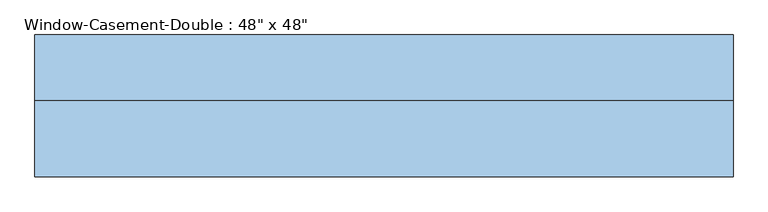
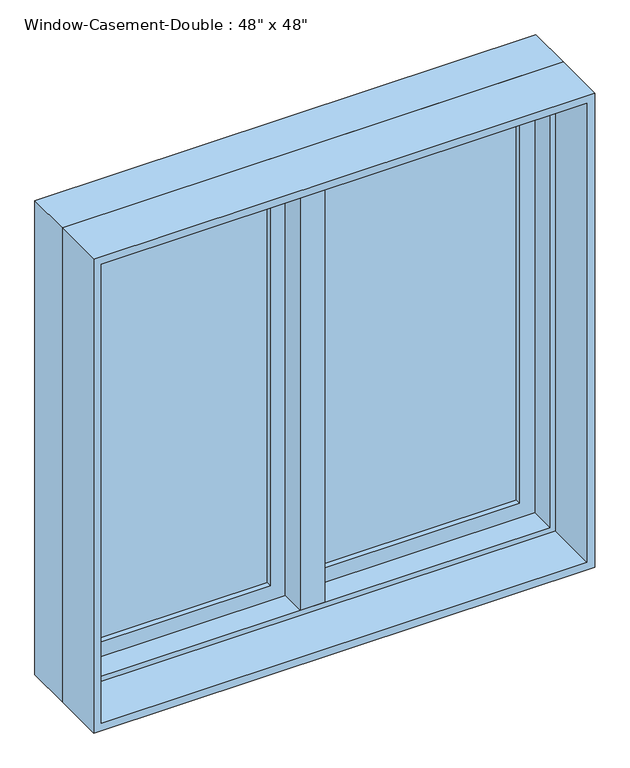
"""IFC4 building model written with IfcOpenShell, lengths in millimetres: window geometry."""

from ifc_helpers import new_model, si_unit, frame, origin, place, context, project, spatial, polyline, outline, extrude, faceted_brep, source, transform, mapped, element, save


def window_9200f5ac(model_context):
    return source(origin(), model_context, "Body", "SolidModel", [
        faceted_brep([(577.85, 82.55, 2101.85), (577.85, 19.05, 2101.85), (-577.85, 19.05, 2101.85), (-577.85, 82.55, 2101.85), (596.9, 133.35, 2120.9), (596.9, 82.55, 2120.9), (-596.9, 82.55, 2120.9), (-596.9, 133.35, 2120.9), (609.6, 19.05, 2133.6), (609.6, 133.35, 2133.6), (-609.6, 133.35, 2133.6), (-609.6, 19.05, 2133.6), (-577.85, 19.05, 946.15), (-577.85, 82.55, 946.15), (-596.9, 82.55, 927.1), (-596.9, 133.35, 927.1), (-609.6, 133.35, 914.4), (-609.6, 19.05, 914.4), (577.85, 19.05, 946.15), (577.85, 82.55, 946.15), (596.9, 82.55, 927.1), (596.9, 133.35, 927.1), (609.6, 133.35, 914.4), (609.6, 19.05, 914.4)], [[[0, 1, 2, 3]], [[4, 5, 6, 7]], [[8, 9, 10, 11]], [[3, 2, 12, 13]], [[7, 6, 14, 15]], [[11, 10, 16, 17]], [[13, 12, 18, 19]], [[15, 14, 20, 21]], [[17, 16, 22, 23]], [[11, 17, 23, 8], [1, 18, 12, 2]], [[19, 18, 1, 0]], [[5, 20, 14, 6], [3, 13, 19, 0]], [[21, 20, 5, 4]], [[23, 22, 9, 8]], [[9, 22, 16, 10], [7, 15, 21, 4]]]),
        extrude(outline(polyline([(2133.6, -609.6), (914.4, -609.6), (914.4, 609.6), (2133.6, 609.6), (2133.6, -609.6)]), holes=[polyline([(2114.55, 590.55), (933.45, 590.55), (933.45, -590.55), (2114.55, -590.55), (2114.55, 590.55)])]), frame((0.0, -114.3, 0.0), z_axis=(0.0, 1.0, 0.0), x_axis=(0.0, 0.0, 1.0)), (0.0, 0.0, 1.0), 133.35),
        extrude(outline(polyline([(927.1, 596.9), (2120.9, 596.9), (2120.9, 9.525), (927.1, 9.525), (927.1, 596.9)]), holes=[polyline([(984.25, 66.675), (2063.75, 66.675), (2063.75, 539.75), (984.25, 539.75), (984.25, 66.675)])]), frame((0.0, 82.55, 0.0), z_axis=(0.0, 1.0, 0.0), x_axis=(0.0, 0.0, 1.0)), (0.0, 0.0, 1.0), 44.45),
        extrude(outline(polyline([(2120.9, -596.9), (927.1, -596.9), (927.1, -9.525), (2120.9, -9.525), (2120.9, -596.9)]), holes=[polyline([(2063.75, -66.675), (984.25, -66.675), (984.25, -539.75), (2063.75, -539.75), (2063.75, -66.675)])]), frame((0.0, 82.55, 0.0), z_axis=(0.0, 1.0, 0.0), x_axis=(0.0, 0.0, 1.0)), (0.0, 0.0, 1.0), 44.45),
        extrude(outline(polyline([(539.75, 114.3), (539.75, 107.95), (66.675, 107.95), (66.675, 114.3), (539.75, 114.3)])), frame((0.0, 0.0, 984.25), z_axis=(0.0, 0.0, 1.0), x_axis=(1.0, 0.0, 0.0)), (0.0, 0.0, 1.0), 1079.5),
        extrude(outline(polyline([(66.675, 95.25), (66.675, 101.6), (539.75, 101.6), (539.75, 95.25), (66.675, 95.25)])), frame((0.0, 0.0, 984.25), z_axis=(0.0, 0.0, 1.0), x_axis=(1.0, 0.0, 0.0)), (0.0, 0.0, 1.0), 1079.5),
        extrude(outline(polyline([(-66.675, 114.3), (-66.675, 107.95), (-539.75, 107.95), (-539.75, 114.3), (-66.675, 114.3)])), frame((0.0, 0.0, 984.25), z_axis=(0.0, 0.0, 1.0), x_axis=(1.0, 0.0, 0.0)), (0.0, 0.0, 1.0), 1079.5),
        extrude(outline(polyline([(-539.75, 95.25), (-539.75, 101.6), (-66.675, 101.6), (-66.675, 95.25), (-539.75, 95.25)])), frame((0.0, 0.0, 984.25), z_axis=(0.0, 0.0, 1.0), x_axis=(1.0, 0.0, 0.0)), (0.0, 0.0, 1.0), 1079.5),
        faceted_brep([(9.525, 133.35, 2120.9), (-9.525, 133.35, 2120.9), (-9.525, 82.55, 2120.9), (9.525, 82.55, 2120.9), (9.525, 133.35, 927.1), (9.525, 82.55, 927.1), (-9.525, 82.55, 927.1), (-9.525, 133.35, 927.1), (-9.525, 82.55, 946.15), (-9.525, 82.55, 2101.85), (-30.1625, 82.55, 946.15), (-30.1625, 82.55, 2101.85), (-30.1625, 19.05, 946.15), (-30.1625, 19.05, 2101.85), (30.1625, 19.05, 946.15), (30.1625, 19.05, 2101.85), (30.1625, 82.55, 946.15), (30.1625, 82.55, 2101.85), (9.525, 82.55, 946.15), (9.525, 82.55, 2101.85)], [[[0, 1, 2, 3]], [[4, 5, 6, 7]], [[1, 0, 4, 7]], [[2, 1, 7, 6, 8, 9]], [[9, 8, 10, 11]], [[11, 10, 12, 13]], [[13, 12, 14, 15]], [[15, 14, 16, 17]], [[17, 16, 18, 19]], [[0, 3, 19, 18, 5, 4]], [[18, 8, 6, 5]], [[9, 19, 3, 2]], [[8, 18, 16, 14, 12, 10]], [[19, 9, 11, 13, 15, 17]]]),
    ])


if __name__ == "__main__":
    model = new_model("IFC4")
    model_context = context("Model", 3, world=origin())
    ifc_project = project(units=[si_unit("LENGTHUNIT", "METRE", prefix="MILLI")], contexts=[model_context])
    site = spatial("IfcSite", under=ifc_project)
    building = spatial("IfcBuilding", under=site)
    placement = place(None, origin())
    window_shape = window_9200f5ac(model_context)
    element("IfcWindow", 1, ObjectType="Window-Casement-Double : 48\" x 48\"", at=placement, inside=building, context=model_context, shape_type="MappedRepresentation", body=[
        mapped(window_shape, transform((0.0, 0.0, 0.0), x_axis=(1.0, 0.0, 0.0), y_axis=(0.0, 1.0, 0.0), z_axis=(0.0, 0.0, 1.0))),
    ])
    save(model, "model.ifc")

# Revit data of these elements
# Type "Window-Casement-Double : 48\" x 48\""
#   Type Mark = "18"
#   Fire Rating = "0.5h"
#   Assembly Code = "B2020100"
#   Analytic Construction = "Double glazing - domestic"
#   Frame Extension [instance default] = 0' - 0 1/4"
#   Window Inset [instance default] = 0' - 0"
#   Wall Thickness [instance default] = 0' - 6"
#   Interior Wall Closure [instance default] = 0' - 2 1/4"
#   Half Width = 2' - 0"
#   Visual Light Transmittance = 0.81
#   Thermal Resistance (R) = 1.8146 (h·ft²·°F)/BTU
#   Solar Heat Gain Coefficient = 0.76
#   Rough Width = 4' - 0 1/2"
#   Rough Height = 4' - 0 1/2"
#   Height = 4' - 0"
#   Heat Transfer Coefficient (U) = 0.5511 BTU/(h·ft²·°F)
#   Exterior Wall Closure [instance default] = 0' - 1 1/4"
#   Extension Jamb [instance default] = 0' - 2 1/4"
#   Default Sill Height = 3' - 0"
#   Width = 4' - 0"
#   Muntin Visibility = yes
#   Interior Trim Visibility [instance default] = yes
#   Exterior Trim Visibility [instance default] = yes
#   Extension Jamb Visibility [instance default] = yes
#   Interior Trim Material = Wood - Stained
#   Muntin Pattern = Muntin Pattern_2x2 : Muntin Pattern_2x2
#   Interior Trim = Trim-Window-Interior-Flat : Picture Frame
#   Interior Frame Material = Wood - Stained
#   Glass Panel Material = Glass
#   Exterior Trim Material = Clad - White
#   Exterior Trim = Trim-Window-Exterior-Flat : with Sill
#   Exterior Frame Material = Clad - White
#   Wall Closure = (empty or 0)
# Element 1 (IfcWindow, "Window-Casement-Double : 48\" x 48\"")
#   Wall Thickness = 0' - 9"
#   Extension Jamb = 0' - 5 1/4"
#   Materials on its faces: "Wood - Stained", "Glass", "Clad - White"
# Materials
#   "Wood - Stained": class "Wood", colour RGB 224 178 126, transparency 0, Cost = 0
#   "Glass": class "Glass", colour RGB 0 128 192, transparency 0.75, Description = "Soda Lime Glass", Cost = 0
#   "Clad - White": class "Wood", colour RGB 242 242 238, transparency 0, Cost = 0
